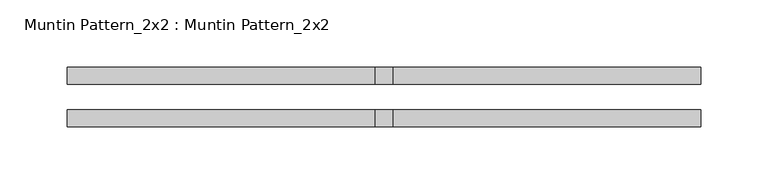
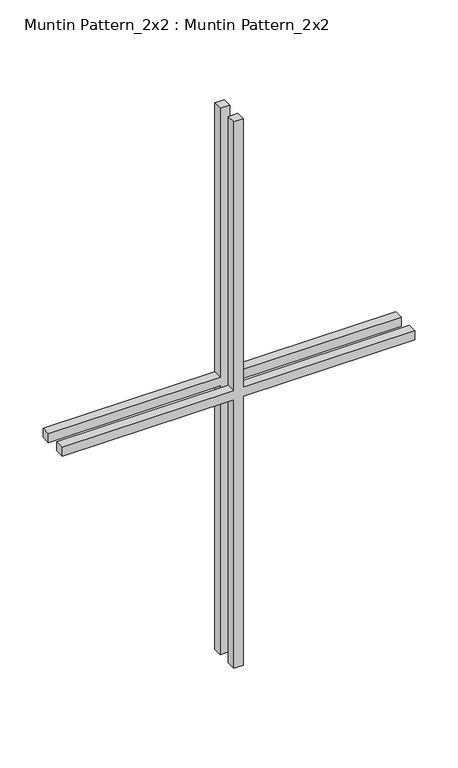
"""IFC4 building model written with IfcOpenShell, lengths in millimetres: proxy geometry, Muntin Pattern_2x2 : Muntin Pattern_2x2."""

from ifc_helpers import new_model, si_unit, frame, origin, place, context, project, spatial, polyline, outline, extrude, source, transform, mapped, element, save


def muntin_pattern_2x2_muntin_pattern_2x2_302d8f29(model_context):
    return source(origin(), model_context, "Body", "SweptSolid", [
        extrude(outline(polyline([(393.7, -6.35), (393.7, -236.5375), (381.0, -236.5375), (381.0, -6.35), (0.0, -6.35), (0.0, 6.35), (381.0, 6.35), (381.0, 236.5375), (393.7, 236.5375), (393.7, 6.35), (774.7, 6.35), (774.7, -6.35), (393.7, -6.35)])), frame((0.0, -22.225, 0.0), z_axis=(0.0, 1.0, 0.0), x_axis=(0.0, 0.0, 1.0)), (0.0, 0.0, 1.0), 12.7),
        extrude(outline(polyline([(393.7, -6.35), (393.7, -236.5375), (381.0, -236.5375), (381.0, -6.35), (0.0, -6.35), (0.0, 6.35), (381.0, 6.35), (381.0, 236.5375), (393.7, 236.5375), (393.7, 6.35), (774.7, 6.35), (774.7, -6.35), (393.7, -6.35)])), frame((0.0, 9.525, 0.0), z_axis=(0.0, 1.0, 0.0), x_axis=(0.0, 0.0, 1.0)), (0.0, 0.0, 1.0), 12.7),
    ])


if __name__ == "__main__":
    model = new_model("IFC4")
    model_context = context("Model", 3, world=origin())
    ifc_project = project(units=[si_unit("LENGTHUNIT", "METRE", prefix="MILLI")], contexts=[model_context])
    site = spatial("IfcSite", under=ifc_project)
    building = spatial("IfcBuilding", under=site)
    placement = place(None, origin())
    muntin_pattern_2x2_muntin_pattern_2x2_shape = muntin_pattern_2x2_muntin_pattern_2x2_302d8f29(model_context)
    element("IfcBuildingElementProxy", 1, Name="Muntin Pattern_2x2 : Muntin Pattern_2x2", ObjectType="Muntin Pattern_2x2 : Muntin Pattern_2x2", at=placement, inside=building, context=model_context, shape_type="MappedRepresentation", body=[
        mapped(muntin_pattern_2x2_muntin_pattern_2x2_shape, transform((0.0, 0.0, 0.0), x_axis=(1.0, 0.0, 0.0), y_axis=(0.0, 1.0, 0.0), z_axis=(0.0, 0.0, 1.0))),
    ])
    save(model, "model.ifc")

# Revit data of these elements
# Type "Muntin Pattern_2x2 : Muntin Pattern_2x2"
#   Width [instance default] = 4' - 0"
#   Thickness = 0' - 0 1/2"
#   Height [instance default] = 4' - 0"
#   Distance = 0' - 0 3/4"
#   Interior Material [instance default] = none
#   Exterior Material [instance default] = none
#   Default Elevation = 0
# Element 1 (IfcBuildingElementProxy, "Muntin Pattern_2x2 : Muntin Pattern_2x2")
#   Width = 1' - 6 5/8"
#   Height = 2' - 6 1/2"
#   Interior Material = Wood - Stained
#   Exterior Material = Clad - White
#   Materials on its faces: "Clad - White", "Wood - Stained"
# Materials
#   "Clad - White": class "Wood", colour RGB 242 242 238, transparency 0, Cost = 0
#   "Wood - Stained": class "Wood", colour RGB 224 178 126, transparency 0, Cost = 0
